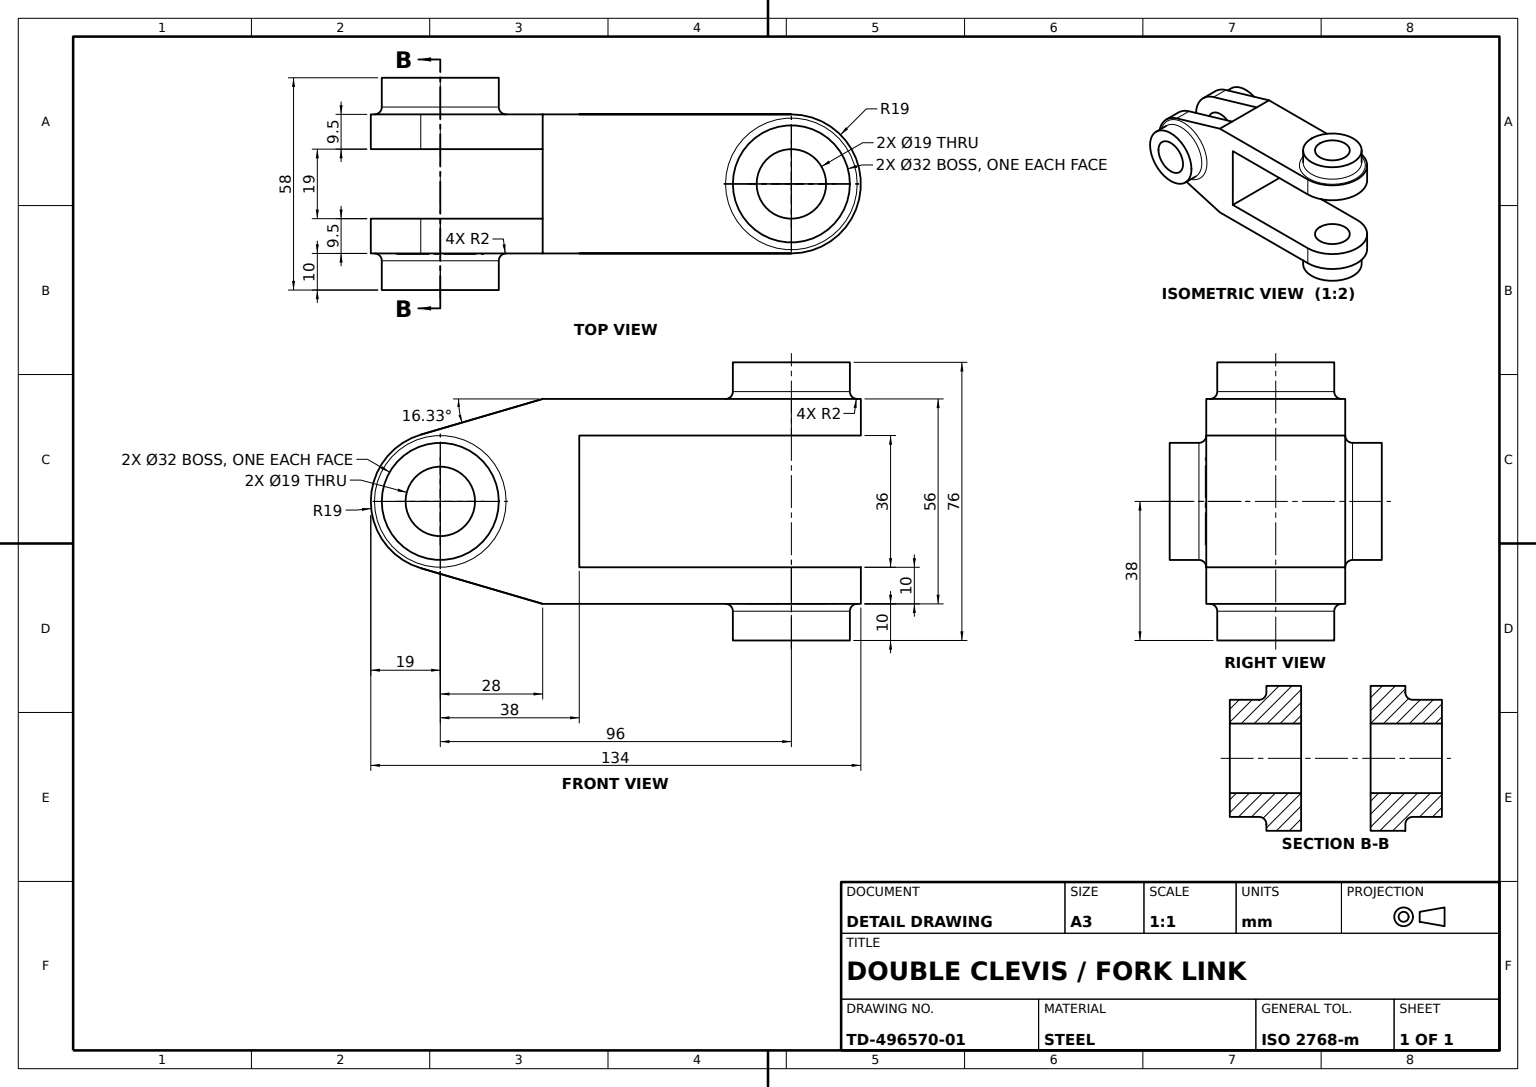
from build123d import *

# Parameters (mm, degrees)
LINK_BODY_PROFILE_SKETCH_R = 9.5
LINK_BODY_38MM_DEPTH       = 19
FORK_END_BOSS_A_SKETCH_R   = 19
FORK_END_BOSS_A_DEPTH      = 10
FORK_START                 = -10
FORK_END_BOSS_B_SKETCH_R   = 19
FORK_END_BOSS_B_DEPTH      = 10
FORK_SLOT_SKETCH_W         = 47
FORK_SLOT_SKETCH_H         = 19
FORK_SLOT_19MM_DEPTH       = 67
SIDE_HUB_SKETCH_32_R       = 16
SIDE_HUB_SKETCH_32_R_2     = 9.5
SIDE_HUB_32_DEPTH          = 10
FORK_HUB_SKETCH_32_R       = 16
FORK_HUB_32_DEPTH          = 10
FORK_PIN_BORE_SKETCH_19_R  = 9.5
FORK_PIN_BORE_19_DEPTH     = 141.861634237
EDGE_FILLETS_R2_R          = 2


with BuildPart() as part:
    # Link Body Profile Sketch → Link Body 38mm (new, symmetric)
    with BuildSketch(Plane.XY):
        with BuildLine():
            Line((-5.341003663, 18.233860806), (28, 28))
            Line((28, 28), (96, 28))
            Line((96, 28), (96, 18))
            Line((96, 18), (38, 18))
            Line((38, 18), (38, -18))
            Line((38, -18), (96, -18))
            Line((96, -18), (96, -28))
            Line((96, -28), (28, -28))
            Line((28, -28), (-5.341003663, -18.233860806))
            ThreePointArc((-5.341003663, -18.233860806), (-19, 0), (-5.341003663, 18.233860806))
        make_face()
        Circle(LINK_BODY_PROFILE_SKETCH_R, mode=Mode.SUBTRACT)
    extrude(amount=LINK_BODY_38MM_DEPTH, both=True)

    # Fork End Boss A Sketch → Fork End Boss A (add)
    with BuildSketch(Plane(origin=(0, 28, 0), x_dir=(1, 0, 0), z_dir=(0, 1, 0))):
        with Locations((96, 0)):
            Circle(FORK_END_BOSS_A_SKETCH_R)
    extrude(amount=-FORK_END_BOSS_A_DEPTH)

    # Fork End Boss B Sketch → Fork End Boss B (add)
    with BuildSketch(Plane.XZ.offset(28).offset(FORK_START)):
        with Locations((96, 0)):
            Circle(FORK_END_BOSS_B_SKETCH_R)
    extrude(amount=FORK_END_BOSS_B_DEPTH)

    # Fork Slot Sketch → Fork Slot 19mm (cut)
    with BuildSketch(Plane.XZ.offset(28)):
        with Locations((4.5, 0)):
            Rectangle(FORK_SLOT_SKETCH_W, FORK_SLOT_SKETCH_H)
    extrude(amount=-FORK_SLOT_19MM_DEPTH, mode=Mode.SUBTRACT)

    # Side Hub Sketch Ø32 → Side Hub Ø32 (add)
    with BuildSketch(Plane.XY.offset(19)):
        Circle(SIDE_HUB_SKETCH_32_R)
        Circle(SIDE_HUB_SKETCH_32_R_2, mode=Mode.SUBTRACT)
    side_hub_32 = extrude(amount=SIDE_HUB_32_DEPTH)

    # Side Hub Mirror: Side Hub Ø32 across plane
    add(side_hub_32.mirror(Plane.XY))

    # Fork Hub Sketch Ø32 → Fork Hub Ø32 (add)
    with BuildSketch(Plane(origin=(0, 28, 0), x_dir=(1, 0, 0), z_dir=(0, 1, 0))):
        with Locations((96, 0)):
            Circle(FORK_HUB_SKETCH_32_R)
    fork_hub_32 = extrude(amount=FORK_HUB_32_DEPTH)

    # Fork Hub Mirror: Fork Hub Ø32 across plane
    add(fork_hub_32.mirror(Plane.ZX))

    # Fork Pin Bore Sketch Ø19 → Fork Pin Bore Ø19 (cut, through all)
    with BuildSketch(Plane.XZ.offset(38)):
        with Locations((96, 0)):
            Circle(FORK_PIN_BORE_SKETCH_19_R)
    extrude(amount=-FORK_PIN_BORE_19_DEPTH, mode=Mode.SUBTRACT)

    # Edge Fillets R2
    edge_fillets_r2_edges = [part.edges().sort_by_distance(p)[0] for p in [
        (80, -28, 0),
        (-16, 0, 19),
        (-16, 0, -19),
        (80, 28, 0),
    ]]
    fillet(edge_fillets_r2_edges, radius=EDGE_FILLETS_R2_R)


solid = part.part
